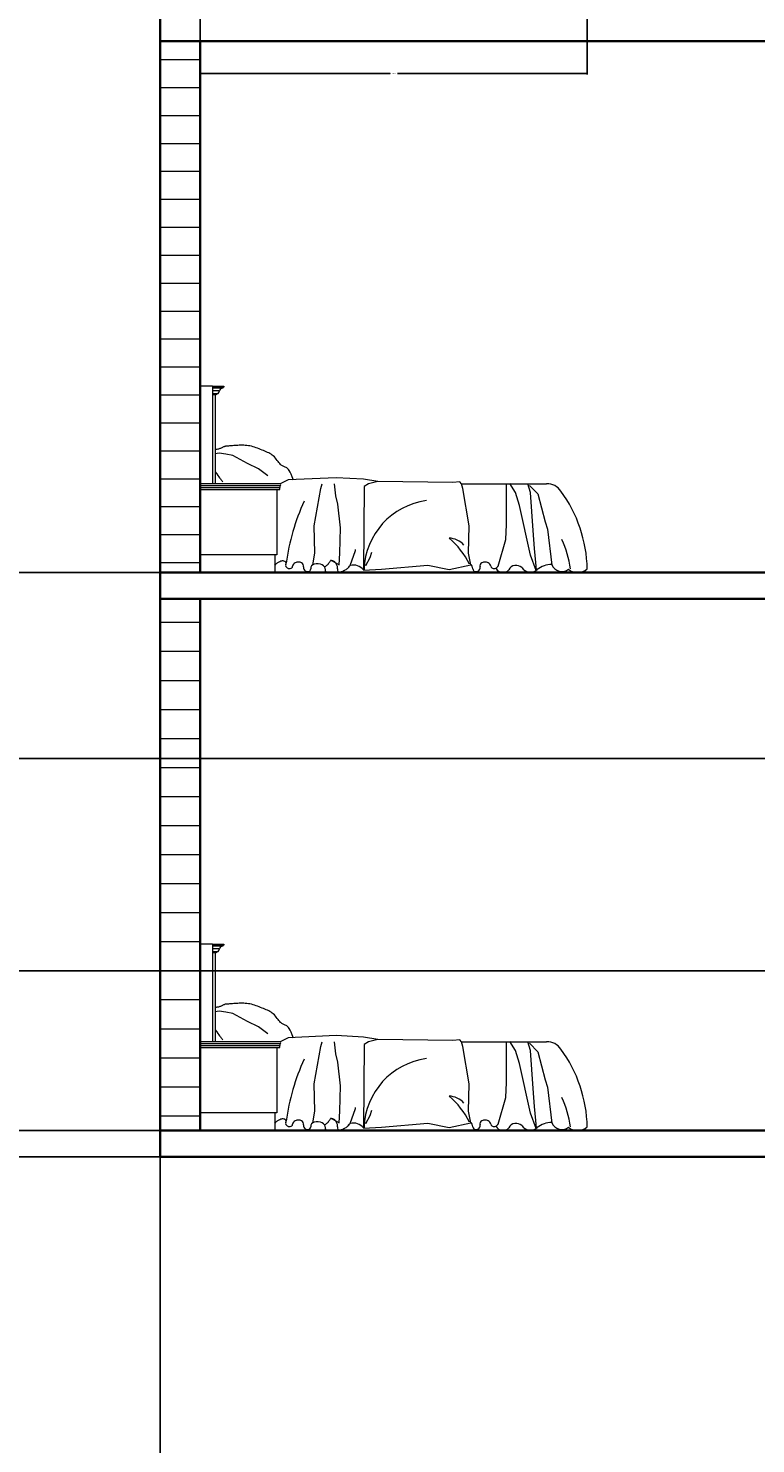
# Model space of a CAD drawing. Units: inches. Extents: x 1355 to 2746, y 1171 to 2751.
# Tile 20 of 24: x 2051 to 2215, y 2155 to 2474. Entities that reach past the tile are written whole.
import ezdxf

# ---------------------------------------------------------------- set-up
doc = ezdxf.new("R2010")
doc.units = ezdxf.units.IN
for name, color, linetype, lineweight in [('A-ANNO-DIMS', 2, 'Continuous', 18), ('A-FURN', 8, 'Continuous', 13), ('A-SECT', 7, 'Continuous', 35), ('A-WALL-PATT', 252, 'Continuous', 13)]:
    doc.layers.add(name, color=color, linetype=linetype, lineweight=lineweight)
doc.styles.get("Standard").update_dxf_attribs({"font": 'arial.ttf'})
doc.dimstyles.get("Standard").update_dxf_attribs({"dimtxt": 0.18, "dimasz": 0.18, "dimexe": 0.18, "dimexo": 0.0625, "dimgap": 0.09, "dimtad": 0, "dimtih": 1, "dimtoh": 1, "dimdec": 4, "dimzin": 0, "dimdsep": 46, "dimtxsty": 'Standard', "dimcen": 0.09, "dimadec": 0, "dimazin": 0, "dimtfac": 1, "dimtdec": 4, "dimtofl": 0, "dimtmove": 0, "dimatfit": 3, "dimfxl": 1, "dimtolj": 1, "dimtzin": 0, "dimarcsym": 0})

# ---------------------------------------------------------------- blocks, each defined once
blk = doc.blocks.new('A$C2FF713C3')
for p, q in [((0, 1050.5), (0, 0.5)), ((70, 1050.5), (0, 1050.5)), ((70, 1050.5), (70, 500.5)), ((70, 1050.5), (133.7, 1050.5)), ((127.4, 1044.2), (70, 1044.2)), ((125.8, 1038), (70, 1038)), ((127.4, 1038), (125.8, 1038)), ((133.7, 1044.2), (127.4, 1044.2)), ((127.4, 1044.2), (127.4, 1038)), ((133.7, 1050.5), (133.7, 1044.2)), ((108.5, 1024.2), (70, 1024.2)), ((91.3, 1006.7), (70, 1006.7)), ((91.3, 1000.5), (70, 1000.5)), ((85, 1000.5), (85, 500.5)), ((97.5, 1006.7), (91.3, 1006.7)), ((91.3, 1006.7), (91.3, 1000.5)), ((87.4, 693.2), (83.6, 693.1)), ((107.4, 672.2), (85.3, 669.2)), ((91.2, 693.6), (87.4, 693.2)), ((95.1, 694.2), (91.2, 693.6)), ((99, 694.9), (95.1, 694.2)), ((102.9, 695.9), (99, 694.9)), ((106.8, 697), (102.9, 695.9)), ((110.7, 698.3), (106.8, 697)), ((144.4, 667.7), (107.4, 672.2)), ((114.5, 699.7), (110.7, 698.3)), ((118.2, 701.2), (114.5, 699.7)), ((121.8, 702.9), (118.2, 701.2)), ((125.3, 704.5), (121.8, 702.9)), ((128.7, 706.1), (125.3, 704.5)), ((131.9, 707.6), (128.7, 706.1)), ((134.9, 709), (131.9, 707.6)), ((137.8, 710.2), (134.9, 709)), ((140.5, 711.1), (137.8, 710.2)), ((143, 711.8), (140.5, 711.1)), ((145.5, 712.2), (143, 711.8)), ((184.4, 660.3), (144.4, 667.7)), ((148, 712.5), (145.5, 712.2)), ((150.6, 712.6), (148, 712.5)), ((153.6, 712.7), (150.6, 712.6)), ((156.9, 712.7), (153.6, 712.7)), ((160.7, 712.8), (156.9, 712.7)), ((165.1, 713), (160.7, 712.8)), ((170.2, 713.4), (165.1, 713)), ((175.9, 713.9), (170.2, 713.4)), ((182.3, 714.4), (175.9, 713.9)), ((189.2, 715), (182.3, 714.4)), ((267.2, 614.5), (184.4, 660.3)), ((196.5, 715.6), (189.2, 715)), ((204.1, 716.2), (196.5, 715.6)), ((212.1, 716.7), (204.1, 716.2)), ((220.3, 717.1), (212.1, 716.7)), ((228.7, 717.3), (220.3, 717.1)), ((237.2, 717.3), (228.7, 717.3)), ((245.8, 717.1), (237.2, 717.3)), ((254.4, 716.7), (245.8, 717.1)), ((263.2, 715.9), (254.4, 716.7)), ((271.9, 714.8), (263.2, 715.9)), ((280.7, 713.3), (271.9, 714.8)), ((289.5, 711.4), (280.7, 713.3)), ((298.2, 709.1), (289.5, 711.4)), ((306.9, 706.4), (298.2, 709.1)), ((315.5, 703.4), (306.9, 706.4)), ((324, 700.1), (315.5, 703.4)), ((332.3, 696.8), (324, 700.1)), ((340.6, 693.4), (332.3, 696.8)), ((348.7, 690), (340.6, 693.4)), ((356.6, 686.7), (348.7, 690)), ((364.3, 683.5), (356.6, 686.7)), ((371.9, 680.4), (364.3, 683.5)), ((379.2, 677.3), (371.9, 680.4)), ((386.3, 674), (379.2, 677.3)), ((393.1, 670.5), (386.3, 674)), ((399.8, 666.5), (393.1, 670.5)), ((406.2, 662.1), (399.8, 666.5)), ((412.3, 657), (406.2, 662.1)), ((418.1, 651.3), (412.3, 657)), ((423.7, 645.1), (418.1, 651.3)), ((429.1, 638.6), (423.7, 645.1)), ((434.2, 632), (429.1, 638.6)), ((84.9, 568), (93.7, 555.7)), ((327.9, 585), (267.2, 614.5)), ((381.3, 544.7), (327.9, 585)), ((439, 625.6), (434.2, 632)), ((443.7, 619.6), (439, 625.6)), ((448.1, 614.1), (443.7, 619.6)), ((452.4, 609.5), (448.1, 614.1)), ((456.4, 605.9), (452.4, 609.5)), ((460.3, 603), (456.4, 605.9)), ((464.2, 600.8), (460.3, 603)), ((468, 599.1), (464.2, 600.8)), ((471.7, 597.6), (468, 599.1)), ((475.6, 596.1), (471.7, 597.6)), ((479.6, 594.4), (475.6, 596.1)), ((483.7, 592.3), (479.6, 594.4)), ((488, 589.7), (483.7, 592.3)), ((492.6, 586), (488, 589.7)), ((497.4, 581), (492.6, 586)), ((502.4, 574.2), (497.4, 581)), ((507.8, 565.1), (502.4, 574.2)), ((513.4, 553.5), (507.8, 565.1)), ((450, 500.5), (0, 500.5)), ((450, 488.5), (0, 488.5)), ((93.7, 555.7), (100.6, 546.3)), ((100.6, 546.3), (105.9, 539)), ((105.9, 539), (110.1, 533.2)), ((110.1, 533.2), (113.9, 528.2)), ((113.9, 528.2), (117.6, 523.3)), ((117.6, 523.3), (121.8, 517.9)), ((121.8, 517.9), (127, 511.4)), ((495.7, 521.8), (450, 500.5)), ((766.6, 534.5), (495.7, 521.8)), ((519.3, 538.8), (513.4, 553.5)), ((525.6, 520.7), (519.3, 538.8)), ((679.4, 472.9), (687.3, 500.5)), ((764.1, 432.4), (757.6, 500.5)), ((919.2, 526), (766.6, 534.5)), ((1001, 512.1), (919.2, 526)), ((923, 485), (919.8, 13.9)), ((947.7, 499.8), (923, 485)), ((1001, 512.1), (947.7, 499.8)), ((1422.2, 508), (1001, 512.1)), ((1463.2, 511.6), (1422.2, 508)), ((1471.1, 500.5), (1463.2, 511.6)), ((1479, 472.9), (1471.1, 500.5)), ((1471.1, 500.5), (1951, 500.5)), ((1725.7, 369.9), (1725.7, 500.5)), ((1776.6, 450.8), (1743.5, 502.3)), ((1861.3, 450.8), (1846, 500.5)), ((1853.9, 491.3), (1901.8, 443.5)), ((448.7, 477.5), (0, 477.5)), ((446.9, 465.5), (0, 465.5)), ((431.9, 465.5), (431.9, 100.5)), ((642.6, 263.3), (679.4, 472.9)), ((775.1, 384.6), (764.1, 432.4)), ((1515.8, 263.3), (1479, 472.9)), ((1798.7, 377.3), (1776.6, 450.8)), ((1876, 237.5), (1861.3, 450.8)), ((1901.8, 443.5), (1942.3, 285.3)), ((789.8, 252.2), (775.1, 384.6)), ((1725.7, 270.6), (1725.7, 369.9)), ((1861.3, 97.8), (1798.7, 377.3)), ((646.3, 108.8), (642.6, 263.3)), ((786.1, 108.8), (789.8, 252.2)), ((1512.2, 108.8), (1515.8, 263.3)), ((1722, 186), (1725.7, 270.6)), ((1942.3, 285.3), (1957, 244.9)), ((1957, 244.9), (1981.3, 42.2)), ((1677.5, 36.3), (1722, 186)), ((1883.4, 134.6), (1876, 237.5)), ((431.9, 100.5), (0, 100.5)), ((419.9, 100.5), (419.9, 0.5)), ((634, 43.7), (646.3, 108.8)), ((782.5, 42.6), (786.1, 108.8)), ((844.9, 39.6), (874.4, 124.2)), ((874.4, 124.2), (875.1, 130)), ((956.4, 83.1), (931.8, 36.9)), ((964.4, 113.4), (956.4, 83.1)), ((1524.4, 43.7), (1512.2, 108.8)), ((1892.4, 12.1), (1861.3, 97.8)), ((1890.7, 57.3), (1883.4, 134.6)), ((0, 0.5), (419.9, 0.5)), ((734.6, 72), (782.5, 42.6)), ((919.8, 13.9), (1021.5, 19.4)), ((1021.5, 19.4), (1282.6, 41.6)), ((1282.6, 41.6), (1401.6, 17.8)), ((1401.6, 17.8), (1524.4, 43.7)), ((1894.7, 13.8), (1890.7, 57.3))]:
    blk.add_line(p, q)
for centre, radius, start, end in [((125, 1021.3), 16.8, 87.42116, 169.92904), ((90, 1023.7), 18.5, 293.7928, 1.50079), ((443.2, 483.7), 8.28, 310.99411, 35.0512), ((447.3, 494.5), 6.6, 294.61118, 65.38882), ((1951, 400.5), 100, 35.83195, 90), ((435.7, 473.3), 13.6, 324.97742, 17.95445), ((1735.3, -117.1), 1261.8, 155.69024, 172.29016), ((1327.7, 3.6), 404.9, 97.57237, 178.02017), ((1396.7, 0.2), 783.8, 1.45705, 35.83195), ((1400.1, 81.1), 112.5, 40.70885, 88.9264), ((1125.8, -139.2), 432.6, 25.56932, 50.29378), ((1449, -72.7), 642.9, 8.37443, 23.73381), ((259.9, 249), 261.9, 307.63119, 310.56693), ((478.1, -13.1), 79.2, 115.93806, 127.15402), ((517.4, -93.9), 169, 111.78143, 115.93806), ((474.5, 13.6), 53.3, 104.37799, 111.78143), ((466.1, 46.3), 19.5, 71.58245, 104.37799), ((464.6, 41.9), 24.2, 42.22901, 71.58245), ((490.7, 39.5), 10.2, 140.3102, 217.27929), ((475.7, 51.9), 9.23, 320.3102, 42.22901), ((513.6, 57), 39, 217.27929, 233.1579), ((500.7, 39.8), 17.5, 233.1579, 256.94088), ((500.6, 39.4), 17.2, 256.94088, 270), ((500.6, 74), 51.8, 270, 277.51528), ((505.3, 38.6), 16, 277.51528, 349.78267), ((546.4, 31.2), 25.7, 114.29273, 169.78267), ((554.4, 13.4), 45.2, 90, 114.29273), ((554.4, 20.7), 37.9, 63.42724, 90), ((562.2, 36.4), 20.3, 346.09021, 63.42724), ((601.7, 26.6), 20.3, 166.09021, 243.58133), ((609.7, 42.8), 38.3, 243.58133, 251.5824), ((612.4, 50.9), 46.9, 251.5824, 258.81111), ((606.5, 21.1), 16.5, 258.81111, 1.75785), ((648.9, 22.4), 25.9, 104.59371, 181.75785), ((658.8, -15.6), 65.2, 63.45814, 104.59371), ((673, 12.8), 33.4, 4.66977, 63.45814), ((674.1, 83.9), 58.7, 296.89415, 314.45228), ((713.3, 7.3), 7.4, 170.64836, 198.63453), ((677.4, 13.2), 29, 350.64836, 4.66977), ((711.6, 6.7), 5.58, 198.63453, 218.42959), ((207.6, 559.5), 724.9, 314.45228, 314.97091), ((575.9, 190.8), 203.8, 314.97091, 315.94905), ((696.8, 73.9), 35.6, 315.94905, 329.81727), ((762.4, 35.7), 40.4, 136.79901, 149.81727), ((740.9, 55.9), 10.9, 81.87802, 136.79901), ((738.1, 36.1), 30.8, 50.07733, 81.87802), ((735.6, 33.1), 34.7, 33.71681, 50.07733), ((690, 2.7), 89.5, 23.5428, 33.71681), ((747.6, 27.8), 26.6, 343.69737, 23.5428), ((788.5, 15.9), 15.9, 163.69737, 216.05798), ((783.9, 12.5), 10.2, 216.05798, 282.98191), ((759.3, 118.9), 119.4, 282.98191, 301.5385), ((783.2, 80.1), 73.8, 301.5385, 318.3377), ((782.8, 80.4), 74.3, 318.3377, 326.7067), ((863.8, -27), 69.2, 36.67542, 105.79154), ((957.7, 57), 57.3, 227.99499, 228.65775), ((1509.5, 22.4), 25.9, 358.24215, 61.16814), ((1551.9, 21.1), 16.5, 178.24215, 281.18889), ((1546, 50.9), 46.9, 281.18889, 288.4176), ((1548.7, 42.8), 38.3, 288.4176, 296.41867), ((1556.8, 26.6), 20.3, 296.41867, 13.90979), ((1596.2, 36.4), 20.3, 116.57276, 193.90979), ((1604, 20.7), 37.9, 90, 116.57276), ((1604, 13.4), 45.2, 65.70727, 90), ((1612, 31.2), 25.7, 10.21733, 65.70727), ((1653.1, 38.6), 16, 190.21733, 262.48472), ((1657.8, 74), 51.8, 262.48472, 270), ((1657.8, 39.4), 17.2, 270, 283.05912), ((1657.7, 39.8), 17.5, 283.05912, 306.8421), ((1704.6, 43.4), 43.5, 208.05971, 320.53056), ((1644.8, 57), 39, 306.8421, 322.72071), ((1667.7, 39.5), 10.2, 322.72071, 344.91412), ((1779.5, -6.4), 46.9, 46.72075, 151.78128), ((1859.7, 59.2), 57.3, 213.23769, 312.00501), ((1983.6, -94.9), 140.5, 91.35454, 127.50961), ((2036.9, 65.4), 60.1, 201.78863, 308.33048), ((2126, 84.9), 84.4, 232.07783, 309.92484)]:
    blk.add_arc(centre, radius, start, end)
blk = doc.blocks.new('*D89')
at = {"layer": 'A-ANNO-DIMS', "color": 0, "lineweight": -2, "transparency": 16777216}
for p, q in [((2089.39, 2477.07), (2089.39, 2463.85)), ((2176.75, 2477.07), (2176.75, 2463.85)), ((2089.57, 2464.03), (2132.25, 2464.03)), ((2176.57, 2464.03), (2133.89, 2464.03))]:
    blk.add_line(p, q, dxfattribs=at)
at = {"layer": 'A-ANNO-DIMS', "color": 0, "transparency": 16777216}
for points in [[(2089.57, 2464.06), (2089.57, 2464), (2089.39, 2464.03)], [(2176.57, 2464.06), (2176.57, 2464), (2176.75, 2464.03)]]:
    blk.add_solid(points, dxfattribs=at)
at = {"layer": 'Defpoints', "color": 0, "transparency": 16777216}
for p in [(2089.39, 2477.13), (2176.75, 2477.13), (2176.75, 2464.03)]:
    blk.add_point(p, dxfattribs=at)
at = {"layer": 'A-ANNO-DIMS', "color": 0, "transparency": 16777216, "insert": (2133.07, 2464.03), "char_height": 0.18, "attachment_point": 5}
blk.add_mtext('\\A1;BED 87 TYP.', dxfattribs=at)
blk = doc.blocks.new('*D99')
at = {"layer": 'A-ANNO-DIMS', "color": 0, "lineweight": -2, "transparency": 16777216}
for p, q in [((2080.39, 2139.36), (2080.39, 2716.58)), ((2080.57, 2716.4), (2152.75, 2716.4)), ((2225.71, 2716.4), (2153.53, 2716.4)), ((2225.89, 2139.36), (2225.89, 2716.58))]:
    blk.add_line(p, q, dxfattribs=at)
at = {"layer": 'A-ANNO-DIMS', "color": 0, "transparency": 16777216}
for points in [[(2080.57, 2716.43), (2080.57, 2716.37), (2080.39, 2716.4)], [(2225.71, 2716.43), (2225.71, 2716.37), (2225.89, 2716.4)]]:
    blk.add_solid(points, dxfattribs=at)
at = {"layer": 'Defpoints', "color": 0, "transparency": 16777216}
for p in [(2225.89, 2716.4), (2080.39, 2139.3), (2225.89, 2139.3)]:
    blk.add_point(p, dxfattribs=at)
at = {"layer": 'A-ANNO-DIMS', "color": 0, "transparency": 16777216, "insert": (2153.14, 2716.4), "char_height": 0.18, "attachment_point": 5}
blk.add_mtext('\\A1;145.5', dxfattribs=at)
blk = doc.blocks.new('*D116')
at = {"layer": 'A-ANNO-DIMS', "color": 0, "lineweight": -2, "transparency": 16777216}
for p, q in [((1976.77, 2477.4), (2648.07, 2477.4)), ((2647.89, 2477.22), (2647.89, 2414.58)), ((2647.89, 2351.58), (2647.89, 2414.22)), ((1976.77, 2351.4), (2648.07, 2351.4))]:
    blk.add_line(p, q, dxfattribs=at)
at = {"layer": 'A-ANNO-DIMS', "color": 0, "transparency": 16777216}
for points in [[(2647.86, 2477.22), (2647.92, 2477.22), (2647.89, 2477.4)], [(2647.86, 2351.58), (2647.92, 2351.58), (2647.89, 2351.4)]]:
    blk.add_solid(points, dxfattribs=at)
at = {"layer": 'Defpoints', "color": 0, "transparency": 16777216}
for p in [(1976.71, 2477.4), (2647.89, 2477.4), (1976.71, 2351.4)]:
    blk.add_point(p, dxfattribs=at)
at = {"layer": 'A-ANNO-DIMS', "color": 0, "transparency": 16777216, "insert": (2647.89, 2414.4), "char_height": 0.18, "attachment_point": 5}
blk.add_mtext('\\A1;126', dxfattribs=at)
blk = doc.blocks.new('*D123')
at = {"layer": 'A-ANNO-DIMS', "color": 0, "lineweight": -2, "transparency": 16777216}
for p, q in [((1880.77, 2261.4), (2648.07, 2261.4)), ((2647.89, 2261.22), (2647.89, 2243.58)), ((2647.89, 2225.58), (2647.89, 2243.22)), ((1940.77, 2225.4), (2648.07, 2225.4))]:
    blk.add_line(p, q, dxfattribs=at)
at = {"layer": 'A-ANNO-DIMS', "color": 0, "transparency": 16777216}
for points in [[(2647.86, 2261.22), (2647.92, 2261.22), (2647.89, 2261.4)], [(2647.86, 2225.58), (2647.92, 2225.58), (2647.89, 2225.4)]]:
    blk.add_solid(points, dxfattribs=at)
at = {"layer": 'Defpoints', "color": 0, "transparency": 16777216}
for p in [(1880.71, 2261.4), (2647.89, 2261.4), (1940.71, 2225.4)]:
    blk.add_point(p, dxfattribs=at)
at = {"layer": 'A-ANNO-DIMS', "color": 0, "transparency": 16777216, "insert": (2647.89, 2243.4), "char_height": 0.18, "attachment_point": 5}
blk.add_mtext('\\A1;36', dxfattribs=at)
blk = doc.blocks.new('*D125')
at = {"layer": 'A-ANNO-DIMS', "color": 0, "lineweight": -2, "transparency": 16777216}
for p, q in [((1880.77, 2309.4), (2648.07, 2309.4)), ((2647.89, 2309.22), (2647.89, 2285.58)), ((2647.89, 2261.58), (2647.89, 2285.22)), ((1880.77, 2261.4), (2648.07, 2261.4))]:
    blk.add_line(p, q, dxfattribs=at)
at = {"layer": 'A-ANNO-DIMS', "color": 0, "transparency": 16777216}
for points in [[(2647.86, 2309.22), (2647.92, 2309.22), (2647.89, 2309.4)], [(2647.86, 2261.58), (2647.92, 2261.58), (2647.89, 2261.4)]]:
    blk.add_solid(points, dxfattribs=at)
at = {"layer": 'Defpoints', "color": 0, "transparency": 16777216}
for p in [(1880.71, 2309.4), (2647.89, 2309.4), (1880.71, 2261.4)]:
    blk.add_point(p, dxfattribs=at)
at = {"layer": 'A-ANNO-DIMS', "color": 0, "transparency": 16777216, "insert": (2647.89, 2285.4), "char_height": 0.18, "attachment_point": 5}
blk.add_mtext('\\A1;48', dxfattribs=at)
blk = doc.blocks.new('*D126')
at = {"layer": 'A-ANNO-DIMS', "color": 0, "lineweight": -2, "transparency": 16777216}
for p, q in [((2080.39, 2219.34), (2080.39, 1171.06)), ((2506.39, 2219.34), (2506.39, 1171.06)), ((2080.57, 1171.24), (2293.1, 1171.24)), ((2506.21, 1171.24), (2293.68, 1171.24))]:
    blk.add_line(p, q, dxfattribs=at)
at = {"layer": 'A-ANNO-DIMS', "color": 0, "transparency": 16777216}
for points in [[(2080.57, 1171.27), (2080.57, 1171.21), (2080.39, 1171.24)], [(2506.21, 1171.27), (2506.21, 1171.21), (2506.39, 1171.24)]]:
    blk.add_solid(points, dxfattribs=at)
at = {"layer": 'Defpoints', "color": 0, "transparency": 16777216}
for p in [(2080.39, 2219.4), (2506.39, 2219.4), (2506.39, 1171.24)]:
    blk.add_point(p, dxfattribs=at)
at = {"layer": 'A-ANNO-DIMS', "color": 0, "transparency": 16777216, "insert": (2293.39, 1171.24), "char_height": 0.18, "attachment_point": 5}
blk.add_mtext('\\A1;426', dxfattribs=at)
blk = doc.blocks.new('*D127')
at = {"layer": 'A-ANNO-DIMS', "color": 0, "lineweight": -2, "transparency": 16777216}
for p, q in [((2080.33, 2645.4), (1407.53, 2645.4)), ((1407.71, 2645.22), (1407.71, 2432.58)), ((1407.71, 2219.58), (1407.71, 2432.22)), ((2080.33, 2219.4), (1407.53, 2219.4))]:
    blk.add_line(p, q, dxfattribs=at)
at = {"layer": 'A-ANNO-DIMS', "color": 0, "transparency": 16777216}
for points in [[(1407.68, 2645.22), (1407.74, 2645.22), (1407.71, 2645.4)], [(1407.68, 2219.58), (1407.74, 2219.58), (1407.71, 2219.4)]]:
    blk.add_solid(points, dxfattribs=at)
at = {"layer": 'Defpoints', "color": 0, "transparency": 16777216}
for p in [(1407.71, 2645.4), (2080.39, 2645.4), (2080.39, 2219.4)]:
    blk.add_point(p, dxfattribs=at)
at = {"layer": 'A-ANNO-DIMS', "color": 0, "transparency": 16777216, "insert": (1407.71, 2432.4), "char_height": 0.18, "attachment_point": 5}
blk.add_mtext('\\A1;426', dxfattribs=at)

msp = doc.modelspace()

# ---------------------------------------------------------------- hatches: boundary and pattern name
at = {"layer": 'A-WALL-PATT'}
h = msp.add_hatch(dxfattribs=at)
h.set_pattern_fill('ANSI31', color=256, scale=1.9874, angle=-45, style=0)
h.paths.add_polyline_path([(2080.3909, 2351.3999), (2089.3909, 2351.3999), (2089.3909, 2471.3999), (2080.3909, 2471.3999)])
h = msp.add_hatch(dxfattribs=at)
h.set_pattern_fill('ANSI31', color=256, scale=2.06457, angle=-45, style=0)
h.paths.add_polyline_path([(2080.3909, 2225.3999), (2089.3909, 2225.3999), (2089.3909, 2345.3999), (2080.3909, 2345.3999)])

# ---------------------------------------------------------------- linework, layer by layer
at = {"layer": 'A-SECT'}
for p, q in [((2080.3909, 2645.3999), (2080.3909, 2471.3999)), ((2080.3909, 2519.3999), (2080.3909, 2345.3999)), ((2506.3909, 2471.3999), (2080.3909, 2471.3999)), ((2089.3909, 2471.3999), (2089.3909, 2351.3999)), ((2080.3909, 2393.3999), (2080.3909, 2219.3999)), ((2506.3909, 2351.3999), (2080.3909, 2351.3999)), ((2506.3909, 2345.3999), (2080.3909, 2345.3999)), ((2089.3909, 2345.3999), (2089.3909, 2225.3999)), ((2089.3909, 2264.4463), (2089.3909, 2269.5522)), ((2080.3909, 2258.8085), (2080.3909, 2264.4463)), ((2089.3909, 2252.7452), (2089.3909, 2258.8085)), ((2080.3909, 2246.4355), (2080.3909, 2252.7452)), ((2089.3909, 2239.5018), (2089.3909, 2246.4355)), ((2080.3909, 2232.6407), (2080.3909, 2239.5018)), ((2506.3909, 2225.3999), (2080.3909, 2225.3999)), ((2506.3909, 2219.3999), (2080.3909, 2219.3999))]:
    msp.add_line(p, q, dxfattribs=at)

# ---------------------------------------------------------------- block references
at = {"layer": 'A-FURN', "xscale": 0.0400677785412672, "yscale": 0.0400677785412672, "zscale": 0.0400677785412672}
for p in [(2089.3909, 2351.3801), (2089.3909, 2225.3801)]:
    msp.add_blockref('A$C2FF713C3', p, dxfattribs=at)

# ---------------------------------------------------------------- dimensions: what is measured, and where the dimension line sits
at = {"layer": 'A-ANNO-DIMS'}
for base, p1, p2, override, picture, middle in [((2225.8909, 2716.3999), (2080.3909, 2139.3018), (2225.8909, 2139.3018), {"dimdec": 1, "dimlfac": 1, "dimrnd": 0, "dimzin": 0, "dimdsep": 46, "dimlunit": 2}, '*D99', (2153.1409, 2716.3999)), ((2506.3909, 1171.2388), (2080.3909, 2219.3999), (2506.3909, 2219.3999), {"dimdec": 0, "dimlfac": 1, "dimrnd": 0, "dimzin": 0, "dimdsep": 46, "dimlunit": 2}, '*D126', (2293.3909, 1171.2388))]:
    dim = msp.add_linear_dim(base=base, p1=p1, p2=p2, dimstyle='Standard', override=override, dxfattribs=at)
    dim.commit()
    dim.dimension.update_dxf_attribs({"geometry": picture, "text_midpoint": middle})
for base, p1, p2, picture, middle in [((1407.7083, 2645.3999), (2080.3909, 2219.3999), (2080.3909, 2645.3999), '*D127', (1407.7083, 2432.3999)), ((2647.886, 2477.3999), (1976.7083, 2351.3999), (1976.7083, 2477.3999), '*D116', (2647.886, 2414.3999)), ((2647.886, 2309.3999), (1880.7083, 2261.3999), (1880.7083, 2309.3999), '*D125', (2647.886, 2285.3999)), ((2647.886, 2261.3999), (1940.7083, 2225.3999), (1880.7083, 2261.3999), '*D123', (2647.886, 2243.3999))]:
    dim = msp.add_linear_dim(base=base, p1=p1, p2=p2, angle=90, dimstyle='Standard', override={"dimdec": 0, "dimlfac": 1, "dimrnd": 0, "dimzin": 0, "dimdsep": 46, "dimlunit": 2}, dxfattribs=at)
    dim.commit()
    dim.dimension.update_dxf_attribs({"geometry": picture, "text_midpoint": middle})
dim = msp.add_linear_dim(base=(2176.7459, 2464.0311), p1=(2089.3909, 2477.1343), p2=(2176.7459, 2477.1343), text='BED <> TYP.', dimstyle='Standard', override={"dimdec": 0, "dimlfac": 1, "dimrnd": 0, "dimzin": 0, "dimdsep": 46, "dimlunit": 2}, dxfattribs=at)
dim.commit()
dim.dimension.update_dxf_attribs({"geometry": '*D89', "text_midpoint": (2133.0684, 2464.0311)})

doc.saveas('drawing.dxf')
